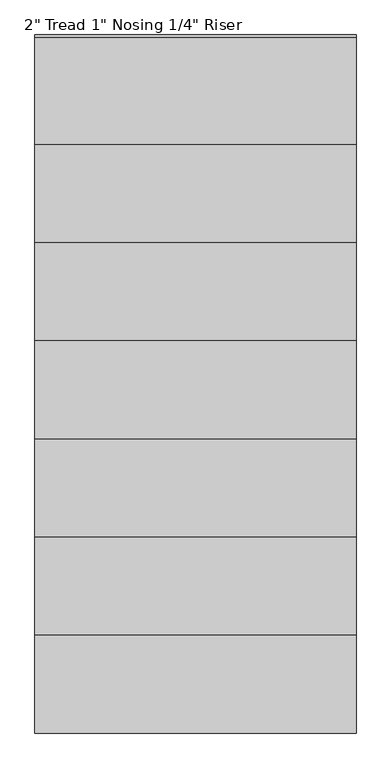
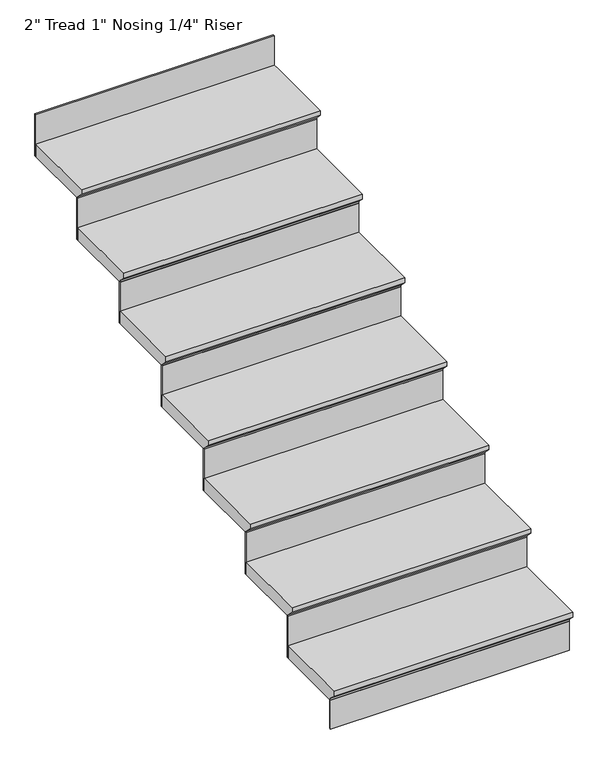
"""IFC4 building model written with IfcOpenShell, lengths in millimetres: stair flight geometry."""

from ifc_helpers import new_model, si_unit, origin, place, context, project, spatial, faceted_brep, source, transform, mapped, element, save


def stair_flight_27979845(model_context):
    return source(origin(), model_context, "Body", "Brep", [
        faceted_brep([(-5380.4481169, -3250.5249317, 759.8833333), (-5380.4481169, -3250.5249317, 778.9333333), (-6294.8481169, -3250.5249317, 778.9333333), (-6294.8481169, -3250.5249317, 759.8833333), (-5380.4481169, -3225.1249317, 734.4833333), (-6294.8481169, -3225.1249317, 734.4833333), (-5380.4481169, -2945.7249317, 778.9333333), (-6294.8481169, -2945.7249317, 778.9333333), (-6294.8481169, -3225.1249317, 728.1333333), (-6294.8481169, -2945.7249317, 728.1333333), (-5380.4481169, -2945.7249317, 728.1333333), (-5380.4481169, -3225.1249317, 728.1333333)], [[[0, 1, 2, 3]], [[4, 0, 3, 5]], [[2, 1, 6, 7]], [[8, 9, 10, 11]], [[2, 7, 9, 8, 5, 3]], [[8, 11, 4, 5]], [[6, 1, 0, 4, 11, 10]], [[7, 6, 10, 9]]]),
        faceted_brep([(-5380.4481169, -3225.1249317, 728.1333333), (-5380.4481169, -3225.1249317, 609.6), (-5380.4481169, -3218.7749317, 609.6), (-5380.4481169, -3218.7749317, 728.1333333), (-6294.8481169, -3225.1249317, 728.1333333), (-6294.8481169, -3218.7749317, 728.1333333), (-6294.8481169, -3218.7749317, 609.6), (-6294.8481169, -3225.1249317, 609.6)], [[[0, 1, 2, 3]], [[4, 5, 6, 7]], [[1, 0, 4, 7]], [[2, 1, 7, 6]], [[3, 2, 6, 5]], [[0, 3, 5, 4]]]),
        faceted_brep([(-5380.4481169, -2945.7249317, 897.4666667), (-5380.4481169, -2945.7249317, 728.1333333), (-5380.4481169, -2939.3749317, 728.1333333), (-5380.4481169, -2939.3749317, 897.4666667), (-6294.8481169, -2945.7249317, 897.4666667), (-6294.8481169, -2939.3749317, 897.4666667), (-6294.8481169, -2939.3749317, 728.1333333), (-6294.8481169, -2945.7249317, 728.1333333)], [[[0, 1, 2, 3]], [[4, 5, 6, 7]], [[1, 0, 4, 7]], [[2, 1, 7, 6]], [[3, 2, 6, 5]], [[0, 3, 5, 4]]]),
        faceted_brep([(-6294.8481169, -2971.1249317, 948.2666667), (-5380.4481169, -2971.1249317, 948.2666667), (-5380.4481169, -2666.3249317, 948.2666667), (-6294.8481169, -2666.3249317, 948.2666667), (-6294.8481169, -2945.7249317, 897.4666667), (-6294.8481169, -2666.3249317, 897.4666667), (-5380.4481169, -2666.3249317, 897.4666667), (-5380.4481169, -2945.7249317, 897.4666667), (-6294.8481169, -2945.7249317, 903.8166667), (-6294.8481169, -2971.1249317, 929.2166667), (-5380.4481169, -2945.7249317, 903.8166667), (-5380.4481169, -2971.1249317, 929.2166667)], [[[0, 1, 2, 3]], [[4, 5, 6, 7]], [[0, 3, 5, 4, 8, 9]], [[4, 7, 10, 8]], [[2, 1, 11, 10, 7, 6]], [[3, 2, 6, 5]], [[11, 1, 0, 9]], [[10, 11, 9, 8]]]),
        faceted_brep([(-5380.4481169, -2666.3249317, 1066.8), (-5380.4481169, -2666.3249317, 897.4666667), (-5380.4481169, -2659.9749317, 897.4666667), (-5380.4481169, -2659.9749317, 1066.8), (-6294.8481169, -2666.3249317, 1066.8), (-6294.8481169, -2659.9749317, 1066.8), (-6294.8481169, -2659.9749317, 897.4666667), (-6294.8481169, -2666.3249317, 897.4666667)], [[[0, 1, 2, 3]], [[4, 5, 6, 7]], [[1, 0, 4, 7]], [[2, 1, 7, 6]], [[3, 2, 6, 5]], [[0, 3, 5, 4]]]),
        faceted_brep([(-6294.8481169, -2691.7249317, 1117.6), (-5380.4481169, -2691.7249317, 1117.6), (-5380.4481169, -2386.9249317, 1117.6), (-6294.8481169, -2386.9249317, 1117.6), (-6294.8481169, -2666.3249317, 1066.8), (-6294.8481169, -2386.9249317, 1066.8), (-5380.4481169, -2386.9249317, 1066.8), (-5380.4481169, -2666.3249317, 1066.8), (-6294.8481169, -2666.3249317, 1073.15), (-6294.8481169, -2691.7249317, 1098.55), (-5380.4481169, -2666.3249317, 1073.15), (-5380.4481169, -2691.7249317, 1098.55)], [[[0, 1, 2, 3]], [[4, 5, 6, 7]], [[0, 3, 5, 4, 8, 9]], [[4, 7, 10, 8]], [[2, 1, 11, 10, 7, 6]], [[3, 2, 6, 5]], [[11, 1, 0, 9]], [[10, 11, 9, 8]]]),
        faceted_brep([(-5380.4481169, -2386.9249317, 1236.1333333), (-5380.4481169, -2386.9249317, 1066.8), (-5380.4481169, -2380.5749317, 1066.8), (-5380.4481169, -2380.5749317, 1236.1333333), (-6294.8481169, -2386.9249317, 1236.1333333), (-6294.8481169, -2380.5749317, 1236.1333333), (-6294.8481169, -2380.5749317, 1066.8), (-6294.8481169, -2386.9249317, 1066.8)], [[[0, 1, 2, 3]], [[4, 5, 6, 7]], [[1, 0, 4, 7]], [[2, 1, 7, 6]], [[3, 2, 6, 5]], [[0, 3, 5, 4]]]),
        faceted_brep([(-6294.8481169, -2412.3249317, 1286.9333333), (-5380.4481169, -2412.3249317, 1286.9333333), (-5380.4481169, -2107.5249317, 1286.9333333), (-6294.8481169, -2107.5249317, 1286.9333333), (-6294.8481169, -2386.9249317, 1236.1333333), (-6294.8481169, -2107.5249317, 1236.1333333), (-5380.4481169, -2107.5249317, 1236.1333333), (-5380.4481169, -2386.9249317, 1236.1333333), (-6294.8481169, -2386.9249317, 1242.4833333), (-6294.8481169, -2412.3249317, 1267.8833333), (-5380.4481169, -2386.9249317, 1242.4833333), (-5380.4481169, -2412.3249317, 1267.8833333)], [[[0, 1, 2, 3]], [[4, 5, 6, 7]], [[0, 3, 5, 4, 8, 9]], [[4, 7, 10, 8]], [[2, 1, 11, 10, 7, 6]], [[3, 2, 6, 5]], [[11, 1, 0, 9]], [[10, 11, 9, 8]]]),
        faceted_brep([(-5380.4481169, -2107.5249317, 1405.4666667), (-5380.4481169, -2107.5249317, 1236.1333333), (-5380.4481169, -2101.1749317, 1236.1333333), (-5380.4481169, -2101.1749317, 1405.4666667), (-6294.8481169, -2107.5249317, 1405.4666667), (-6294.8481169, -2101.1749317, 1405.4666667), (-6294.8481169, -2101.1749317, 1236.1333333), (-6294.8481169, -2107.5249317, 1236.1333333)], [[[0, 1, 2, 3]], [[4, 5, 6, 7]], [[1, 0, 4, 7]], [[2, 1, 7, 6]], [[3, 2, 6, 5]], [[0, 3, 5, 4]]]),
        faceted_brep([(-6294.8481169, -2132.9249317, 1456.2666667), (-5380.4481169, -2132.9249317, 1456.2666667), (-5380.4481169, -1828.1249317, 1456.2666667), (-6294.8481169, -1828.1249317, 1456.2666667), (-6294.8481169, -2107.5249317, 1405.4666667), (-6294.8481169, -1828.1249317, 1405.4666667), (-5380.4481169, -1828.1249317, 1405.4666667), (-5380.4481169, -2107.5249317, 1405.4666667), (-6294.8481169, -2107.5249317, 1411.8166667), (-6294.8481169, -2132.9249317, 1437.2166667), (-5380.4481169, -2107.5249317, 1411.8166667), (-5380.4481169, -2132.9249317, 1437.2166667)], [[[0, 1, 2, 3]], [[4, 5, 6, 7]], [[0, 3, 5, 4, 8, 9]], [[4, 7, 10, 8]], [[2, 1, 11, 10, 7, 6]], [[3, 2, 6, 5]], [[11, 1, 0, 9]], [[10, 11, 9, 8]]]),
        faceted_brep([(-5380.4481169, -1828.1249317, 1574.8), (-5380.4481169, -1828.1249317, 1405.4666667), (-5380.4481169, -1821.7749317, 1405.4666667), (-5380.4481169, -1821.7749317, 1574.8), (-6294.8481169, -1828.1249317, 1574.8), (-6294.8481169, -1821.7749317, 1574.8), (-6294.8481169, -1821.7749317, 1405.4666667), (-6294.8481169, -1828.1249317, 1405.4666667)], [[[0, 1, 2, 3]], [[4, 5, 6, 7]], [[1, 0, 4, 7]], [[2, 1, 7, 6]], [[3, 2, 6, 5]], [[0, 3, 5, 4]]]),
        faceted_brep([(-6294.8481169, -1853.5249317, 1625.6), (-5380.4481169, -1853.5249317, 1625.6), (-5380.4481169, -1548.7249317, 1625.6), (-6294.8481169, -1548.7249317, 1625.6), (-6294.8481169, -1828.1249317, 1574.8), (-6294.8481169, -1548.7249317, 1574.8), (-5380.4481169, -1548.7249317, 1574.8), (-5380.4481169, -1828.1249317, 1574.8), (-6294.8481169, -1828.1249317, 1581.15), (-6294.8481169, -1853.5249317, 1606.55), (-5380.4481169, -1828.1249317, 1581.15), (-5380.4481169, -1853.5249317, 1606.55)], [[[0, 1, 2, 3]], [[4, 5, 6, 7]], [[0, 3, 5, 4, 8, 9]], [[4, 7, 10, 8]], [[2, 1, 11, 10, 7, 6]], [[3, 2, 6, 5]], [[11, 1, 0, 9]], [[10, 11, 9, 8]]]),
        faceted_brep([(-5380.4481169, -1269.3249317, 1913.4666667), (-5380.4481169, -1269.3249317, 1744.1333333), (-5380.4481169, -1262.9749317, 1744.1333333), (-5380.4481169, -1262.9749317, 1913.4666667), (-6294.8481169, -1269.3249317, 1913.4666667), (-6294.8481169, -1262.9749317, 1913.4666667), (-6294.8481169, -1262.9749317, 1744.1333333), (-6294.8481169, -1269.3249317, 1744.1333333)], [[[0, 1, 2, 3]], [[4, 5, 6, 7]], [[1, 0, 4, 7]], [[2, 1, 7, 6]], [[3, 2, 6, 5]], [[0, 3, 5, 4]]]),
        faceted_brep([(-5380.4481169, -1548.7249317, 1744.1333333), (-5380.4481169, -1548.7249317, 1574.8), (-5380.4481169, -1542.3749317, 1574.8), (-5380.4481169, -1542.3749317, 1744.1333333), (-6294.8481169, -1548.7249317, 1744.1333333), (-6294.8481169, -1542.3749317, 1744.1333333), (-6294.8481169, -1542.3749317, 1574.8), (-6294.8481169, -1548.7249317, 1574.8)], [[[0, 1, 2, 3]], [[4, 5, 6, 7]], [[1, 0, 4, 7]], [[2, 1, 7, 6]], [[3, 2, 6, 5]], [[0, 3, 5, 4]]]),
        faceted_brep([(-6294.8481169, -1574.1249317, 1794.9333333), (-5380.4481169, -1574.1249317, 1794.9333333), (-5380.4481169, -1294.7249317, 1794.9333333), (-5380.4481169, -1269.3249317, 1794.9333333), (-6294.8481169, -1269.3249317, 1794.9333333), (-6294.8481169, -1548.7249317, 1744.1333333), (-6294.8481169, -1269.3249317, 1744.1333333), (-5380.4481169, -1269.3249317, 1744.1333333), (-5380.4481169, -1294.7249317, 1744.1333333), (-5380.4481169, -1548.7249317, 1744.1333333), (-6294.8481169, -1548.7249317, 1750.4833333), (-6294.8481169, -1574.1249317, 1775.8833333), (-5380.4481169, -1548.7249317, 1750.4833333), (-5380.4481169, -1574.1249317, 1775.8833333)], [[[0, 1, 2, 3, 4]], [[5, 6, 7, 8, 9]], [[0, 4, 6, 5, 10, 11]], [[5, 9, 12, 10]], [[2, 1, 13, 12, 9, 8]], [[3, 2, 8, 7]], [[4, 3, 7, 6]], [[13, 1, 0, 11]], [[12, 13, 11, 10]]]),
    ])


if __name__ == "__main__":
    model = new_model("IFC4")
    model_context = context("Model", 3, world=origin())
    ifc_project = project(units=[si_unit("LENGTHUNIT", "METRE", prefix="MILLI")], contexts=[model_context])
    site = spatial("IfcSite", under=ifc_project)
    building = spatial("IfcBuilding", under=site)
    placement = place(None, origin())
    stair_flight_shape = stair_flight_27979845(model_context)
    element("IfcStairFlight", 1, ObjectType="2\" Tread 1\" Nosing 1/4\" Riser", at=placement, inside=building, context=model_context, shape_type="MappedRepresentation", body=[
        mapped(stair_flight_shape, transform((0.0, 0.0, 0.0), x_axis=(1.0, 0.0, 0.0), y_axis=(0.0, 1.0, 0.0), z_axis=(0.0, 0.0, 1.0))),
    ])
    save(model, "model.ifc")
